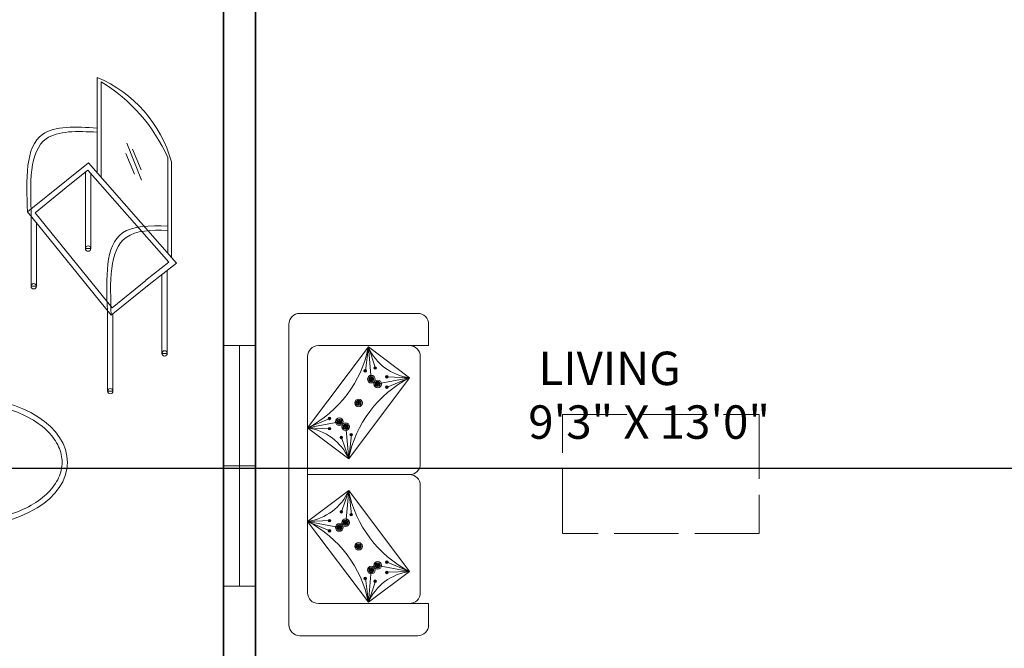
# Model space of a CAD drawing. Units: inches. Extents: x -61 to 1599, y -1316 to 257.
# Tile 19 of 204: x 76 to 259, y -907 to -790. Entities that reach past the tile are written whole.
import ezdxf

# ---------------------------------------------------------------- set-up
doc = ezdxf.new("R2010")
doc.units = ezdxf.units.IN
doc.header["$MEASUREMENT"] = 0
doc.linetypes.add('ACAD_ISO02W100', pattern=[15, 12, -3])
for name, color, linetype, lineweight in [('A-ANNO-DIMS', 2, 'Continuous', 18), ('A-AREA-IDEN', 1, 'Continuous', 18), ('A-FURN-LOW', 83, 'ACAD_ISO02W100', 18), ('FURNITURE', 83, 'Continuous', 18), ('WALLS', 4, 'Continuous', 35), ('WINDOWS', 220, 'Continuous', 18)]:
    doc.layers.add(name, color=color, linetype=linetype, lineweight=lineweight)
doc.layers.add('FUR', color=83, linetype='Continuous')
doc.styles.get("Standard").update_dxf_attribs({"font": 'arial.ttf'})
doc.dimstyles.get("Standard").update_dxf_attribs({"dimtxt": 0.18, "dimasz": 0.18, "dimexe": 0.18, "dimexo": 0.0625, "dimgap": 0.09, "dimtad": 0, "dimtih": 1, "dimtoh": 1, "dimdec": 0, "dimzin": 0, "dimdsep": 46, "dimlunit": 3, "dimtxsty": 'Standard', "dimcen": 0.09, "dimadec": 0, "dimazin": 0, "dimtfac": 1, "dimtdec": 0, "dimtofl": 0, "dimtmove": 0, "dimatfit": 3, "dimfxl": 1, "dimtolj": 1, "dimtzin": 0, "dimarcsym": 0})

# ---------------------------------------------------------------- blocks, each defined once
blk = doc.blocks.new('WIN-45IN')
for p, q in [((0, 44.83), (6, 44.83)), ((0, 0), (6, 0))]:
    blk.add_line(p, q)
for points in [[(6, 44.83), (3, 44.83), (3, 22.42), (6, 22.42)], [(3, 22.42), (0, 22.42), (0, 0), (3, 0)]]:
    blk.add_lwpolyline(points, close=True)
blk = doc.blocks.new('LOUNGE-CHAIR')
for p, q in [((14.76, 41.14), (14.76, 58.89)), ((14.04, 40.33), (14.04, 58.08)), ((6.52, 39.78), (9.29, 46.65)), ((6.58, 41.68), (8.18, 45.54)), ((7.84, 40.87), (9.45, 44.74)), ((0, 24.35), (16.38, 42.98)), ((0.97, 25.45), (0.97, 43.2)), ((0.97, 25.45), (0.97, 43.2)), ((1.64, 26.22), (1.64, 43.97)), ((16.38, 42.98), (20.51, 39.74)), ((16.97, 42.52), (16.97, 42.52)), ((1.45, 24.49), (16.5, 41.61)), ((15.97, 27.05), (15.97, 41.01)), ((16.5, 41.61), (19.89, 38.96)), ((16.97, 27.05), (16.97, 41.25)), ((19.88, 38.97), (26.35, 33.72)), ((20.51, 39.74), (27.76, 33.87)), ((12.02, 16.03), (26.35, 33.72)), ((12.16, 14.63), (27.76, 33.87)), ((27.1, 20.02), (27.1, 33.05)), ((26.1, 20.02), (26.1, 31.82)), ((16.97, 27.05), (15.97, 27.05)), ((0, 24.35), (5.1, 20.35)), ((1.45, 24.49), (5.72, 21.14)), ((0.75, 23.69), (0.79, 23.74)), ((1.73, 7.53), (1.73, 23)), ((2.73, 7.53), (2.73, 22.21)), ((5.1, 20.35), (12.16, 14.63)), ((5.73, 21.13), (12.02, 16.03)), ((27.1, 20.02), (26.1, 20.02)), ((11.85, 0.5), (11.85, 14.88)), ((12.85, 0.5), (12.85, 15.48)), ((2.73, 7.53), (1.73, 7.53)), ((12.85, 0.5), (11.85, 0.5))]:
    blk.add_line(p, q)
for centre in [(16.47, 27.05), (26.6, 20.02), (2.23, 7.53), (12.35, 0.5)]:
    blk.add_circle(centre, 0.5)
for centre, radius, start, end in [((23.93, 36.92), 23.8, 112.6586, 164.6996), ((30.25, 31.33), 31.28, 121.203, 156.1552)]:
    blk.add_arc(centre, radius, start, end)
for points, knots in [([(14.76, 49.49), (18.73, 49.7), (28.38, 50.23), (27.99, 39.93), (27.76, 33.87)], [0, 0, 0, 0, 10.281855, 24.983674, 24.983674, 24.983674, 24.983674]), ([(14.76, 48.72), (18.48, 48.91), (27.65, 49.16), (27.27, 39.12), (27.05, 33.06), (27.04, 33.03), (27.04, 33.01), (27.04, 32.98)], [0.614676, 0.614676, 0.614676, 0.614676, 10.281855, 24.983674, 24.983674, 24.983674, 25.041855, 25.041855, 25.041855, 25.041855]), ([(1.64, 31.22), (4.99, 31.37), (13.47, 31.24), (13.11, 21.57), (12.88, 15.51)], [1.527723, 1.527723, 1.527723, 1.527723, 10.281855, 24.983674, 24.983674, 24.983674, 24.983674]), ([(1.64, 30.44), (4.72, 30.55), (12.75, 30.17), (12.39, 20.76), (12.17, 14.7), (12.16, 14.67), (12.16, 14.65), (12.16, 14.63)], [2.150702, 2.150702, 2.150702, 2.150702, 10.281855, 24.983674, 24.983674, 24.983674, 25.041855, 25.041855, 25.041855, 25.041855])]:
    blk.add_open_spline(points, degree=3, knots=knots)
blk = doc.blocks.new('SIDE-TABLE-OVAL')
blk.add_ellipse((18.95, 11.99), major_axis=(-18.95, 0.16), ratio=0.632617)
blk.add_open_spline([(1, 12.14), (0.99, 11.17), (1.2, 10.2), (2.05, 8.28), (2.69, 7.34), (4.41, 5.58), (5.48, 4.76), (7.96, 3.32), (9.37, 2.71), (12.41, 1.74), (14.05, 1.4), (17.41, 1), (19.13, 0.95), (22.53, 1.15), (24.2, 1.41), (27.36, 2.19), (28.84, 2.73), (31.49, 4.02), (32.66, 4.78), (34.59, 6.45), (35.35, 7.36), (36.44, 9.24), (36.76, 10.2), (36.97, 12.14), (36.87, 13.11), (36.22, 15.04), (35.67, 16), (34.15, 17.81), (33.17, 18.67), (30.85, 20.19), (29.51, 20.86), (26.58, 21.94), (24.98, 22.36), (21.67, 22.89), (19.95, 23.01), (16.54, 22.94), (14.84, 22.76), (11.61, 22.1), (10.07, 21.63), (7.28, 20.44), (6.03, 19.73), (3.92, 18.13), (3.06, 17.25), (1.78, 15.4), (1.35, 14.44), (1.05, 13.03), (1, 12.59), (1, 12.14)], degree=3, knots=[0, 0, 0, 0, 0.279765, 0.279765, 0.559529, 0.559529, 0.839294, 0.839294, 1.119059, 1.119059, 1.398823, 1.398823, 1.678588, 1.678588, 1.958353, 1.958353, 2.238118, 2.238118, 2.517882, 2.517882, 2.797647, 2.797647, 3.077412, 3.077412, 3.357176, 3.357176, 3.636941, 3.636941, 3.916706, 3.916706, 4.19647, 4.19647, 4.476235, 4.476235, 4.756, 4.756, 5.035764, 5.035764, 5.315529, 5.315529, 5.595294, 5.595294, 5.875058, 5.875058, 6.154823, 6.154823, 6.283185, 6.283185, 6.283185, 6.283185])
blk = doc.blocks.new('*U160')
at = {"layer": 'FUR'}
blk.add_open_spline([(0, 0.08), (-0.03, 0.05), (-0.1, -0.02), (0.08, -0.02), (0.02, -0.06), (0, -0.08)], degree=3, knots=[0, 0, 0, 0, 0.0954578, 0.1898773, 0.2470677, 0.2470677, 0.2470677, 0.2470677], dxfattribs=at)
blk = doc.blocks.new('*U161')
at = {"layer": 'FUR', "transparency": 16777216}
for p, rotation in [((222.17, -79.98), 60), ((222.18, -80.06), 120), ((222.31, -79.97), 300), ((222.25, -80.09), 180), ((222.32, -80.05), 240)]:
    blk.add_blockref('*U160', p, dxfattribs=dict(at, rotation=rotation))
blk.add_blockref('*U160', (222.24, -79.93), dxfattribs=at)
blk = doc.blocks.new('*U172')
at = {"layer": 'FUR'}
blk.add_open_spline([(0, 0.08), (-0.03, 0.05), (-0.1, -0.02), (0.08, -0.02), (0.02, -0.06), (0, -0.08)], degree=3, knots=[0, 0, 0, 0, 0.0954578, 0.1898773, 0.2470677, 0.2470677, 0.2470677, 0.2470677], dxfattribs=at)
blk = doc.blocks.new('*U173')
at = {"layer": 'FUR', "transparency": 16777216}
for p, rotation in [((222.17, -79.98), 60), ((222.18, -80.06), 120), ((222.31, -79.97), 300), ((222.25, -80.09), 180), ((222.32, -80.05), 240)]:
    blk.add_blockref('*U172', p, dxfattribs=dict(at, rotation=rotation))
blk.add_blockref('*U172', (222.24, -79.93), dxfattribs=at)
blk = doc.blocks.new('*U186')
at = {"layer": 'FUR'}
blk.add_open_spline([(0, 0.08), (-0.03, 0.05), (-0.1, -0.02), (0.08, -0.02), (0.02, -0.06), (0, -0.08)], degree=3, knots=[0, 0, 0, 0, 0.0954578, 0.1898773, 0.2470677, 0.2470677, 0.2470677, 0.2470677], dxfattribs=at)
blk = doc.blocks.new('*U187')
at = {"layer": 'FUR', "transparency": 16777216}
for p, rotation in [((222.17, -79.98), 60), ((222.18, -80.06), 120), ((222.31, -79.97), 300), ((222.25, -80.09), 180), ((222.32, -80.05), 240)]:
    blk.add_blockref('*U186', p, dxfattribs=dict(at, rotation=rotation))
blk.add_blockref('*U186', (222.24, -79.93), dxfattribs=at)
blk = doc.blocks.new('*U198')
at = {"layer": 'FUR'}
blk.add_open_spline([(0, 0.08), (-0.03, 0.05), (-0.1, -0.02), (0.08, -0.02), (0.02, -0.06), (0, -0.08)], degree=3, knots=[0, 0, 0, 0, 0.0954578, 0.1898773, 0.2470677, 0.2470677, 0.2470677, 0.2470677], dxfattribs=at)
blk = doc.blocks.new('*U199')
at = {"layer": 'FUR', "transparency": 16777216}
for p, rotation in [((222.17, -79.98), 60), ((222.18, -80.06), 120), ((222.31, -79.97), 300), ((222.25, -80.09), 180), ((222.32, -80.05), 240)]:
    blk.add_blockref('*U198', p, dxfattribs=dict(at, rotation=rotation))
blk.add_blockref('*U198', (222.24, -79.93), dxfattribs=at)
blk = doc.blocks.new('*U184')
at = {"layer": 'FUR'}
blk.add_open_spline([(0.01, 0.24), (-0.09, 0.14), (-0.29, -0.05), (0.22, -0.05), (0.07, -0.19), (0.01, -0.24)], degree=3, knots=[0, 0, 0, 0, 0.2846533, 0.5662105, 0.736751, 0.736751, 0.736751, 0.736751], dxfattribs=at)
blk = doc.blocks.new('*U159')
at = {"layer": 'FUR', "transparency": 16777216}
for p, rotation in [((662.52, -238.49), 60), ((662.93, -238.46), 300), ((662.53, -238.73), 120), ((662.74, -238.83), 180), ((662.94, -238.7), 240)]:
    blk.add_blockref('*U184', p, dxfattribs=dict(at, rotation=rotation))
blk.add_blockref('*U184', (662.72, -238.36), dxfattribs=at)
blk = doc.blocks.new('*U210')
at = {"layer": 'FUR'}
blk.add_open_spline([(0.01, 0.24), (-0.09, 0.14), (-0.29, -0.05), (0.22, -0.05), (0.07, -0.19), (0.01, -0.24)], degree=3, knots=[0, 0, 0, 0, 0.2846533, 0.5662105, 0.736751, 0.736751, 0.736751, 0.736751], dxfattribs=at)
blk = doc.blocks.new('*U185')
at = {"layer": 'FUR', "transparency": 16777216}
for p, rotation in [((662.52, -238.49), 60), ((662.93, -238.46), 300), ((662.53, -238.73), 120), ((662.74, -238.83), 180), ((662.94, -238.7), 240)]:
    blk.add_blockref('*U210', p, dxfattribs=dict(at, rotation=rotation))
blk.add_blockref('*U210', (662.72, -238.36), dxfattribs=at)
blk = doc.blocks.new('*U174')
at = {"layer": 'FUR'}
blk.add_open_spline([(0, 0.08), (-0.03, 0.05), (-0.1, -0.02), (0.08, -0.02), (0.02, -0.06), (0, -0.08)], degree=3, knots=[0, 0, 0, 0, 0.0954578, 0.1898773, 0.2470677, 0.2470677, 0.2470677, 0.2470677], dxfattribs=at)
blk = doc.blocks.new('*U175')
at = {"layer": 'FUR', "transparency": 16777216}
for p, rotation in [((222.17, -79.98), 60), ((222.18, -80.06), 120), ((222.31, -79.97), 300), ((222.25, -80.09), 180), ((222.32, -80.05), 240)]:
    blk.add_blockref('*U174', p, dxfattribs=dict(at, rotation=rotation))
blk.add_blockref('*U174', (222.24, -79.93), dxfattribs=at)
blk = doc.blocks.new('*U200')
at = {"layer": 'FUR'}
blk.add_open_spline([(0, 0.08), (-0.03, 0.05), (-0.1, -0.02), (0.08, -0.02), (0.02, -0.06), (0, -0.08)], degree=3, knots=[0, 0, 0, 0, 0.0954578, 0.1898773, 0.2470677, 0.2470677, 0.2470677, 0.2470677], dxfattribs=at)
blk = doc.blocks.new('*U201')
at = {"layer": 'FUR', "transparency": 16777216}
for p, rotation in [((222.17, -79.98), 60), ((222.18, -80.06), 120), ((222.31, -79.97), 300), ((222.25, -80.09), 180), ((222.32, -80.05), 240)]:
    blk.add_blockref('*U200', p, dxfattribs=dict(at, rotation=rotation))
blk.add_blockref('*U200', (222.24, -79.93), dxfattribs=at)
blk = doc.blocks.new('*U168')
at = {"layer": 'FUR'}
blk.add_open_spline([(0.01, 0.24), (-0.09, 0.14), (-0.29, -0.05), (0.22, -0.05), (0.07, -0.19), (0.01, -0.24)], degree=3, knots=[0, 0, 0, 0, 0.2846533, 0.5662105, 0.736751, 0.736751, 0.736751, 0.736751], dxfattribs=at)
blk = doc.blocks.new('*U169')
at = {"layer": 'FUR', "transparency": 16777216}
for p, rotation in [((662.52, -238.49), 60), ((662.93, -238.46), 300), ((662.53, -238.73), 120), ((662.74, -238.83), 180), ((662.94, -238.7), 240)]:
    blk.add_blockref('*U168', p, dxfattribs=dict(at, rotation=rotation))
blk.add_blockref('*U168', (662.72, -238.36), dxfattribs=at)
blk = doc.blocks.new('*U194')
at = {"layer": 'FUR'}
blk.add_open_spline([(0.01, 0.24), (-0.09, 0.14), (-0.29, -0.05), (0.22, -0.05), (0.07, -0.19), (0.01, -0.24)], degree=3, knots=[0, 0, 0, 0, 0.2846533, 0.5662105, 0.736751, 0.736751, 0.736751, 0.736751], dxfattribs=at)
blk = doc.blocks.new('*U195')
at = {"layer": 'FUR', "transparency": 16777216}
for p, rotation in [((662.52, -238.49), 60), ((662.93, -238.46), 300), ((662.53, -238.73), 120), ((662.74, -238.83), 180), ((662.94, -238.7), 240)]:
    blk.add_blockref('*U194', p, dxfattribs=dict(at, rotation=rotation))
blk.add_blockref('*U194', (662.72, -238.36), dxfattribs=at)
blk = doc.blocks.new('*U176')
at = {"layer": 'FUR'}
blk.add_open_spline([(0, 0.08), (-0.03, 0.05), (-0.1, -0.02), (0.08, -0.02), (0.02, -0.06), (0, -0.08)], degree=3, knots=[0, 0, 0, 0, 0.0954578, 0.1898773, 0.2470677, 0.2470677, 0.2470677, 0.2470677], dxfattribs=at)
blk = doc.blocks.new('*U177')
at = {"layer": 'FUR', "transparency": 16777216}
for p, rotation in [((222.17, -79.98), 60), ((222.18, -80.06), 120), ((222.31, -79.97), 300), ((222.25, -80.09), 180), ((222.32, -80.05), 240)]:
    blk.add_blockref('*U176', p, dxfattribs=dict(at, rotation=rotation))
blk.add_blockref('*U176', (222.24, -79.93), dxfattribs=at)
blk = doc.blocks.new('*U202')
at = {"layer": 'FUR'}
blk.add_open_spline([(0, 0.08), (-0.03, 0.05), (-0.1, -0.02), (0.08, -0.02), (0.02, -0.06), (0, -0.08)], degree=3, knots=[0, 0, 0, 0, 0.0954578, 0.1898773, 0.2470677, 0.2470677, 0.2470677, 0.2470677], dxfattribs=at)
blk = doc.blocks.new('*U203')
at = {"layer": 'FUR', "transparency": 16777216}
for p, rotation in [((222.17, -79.98), 60), ((222.18, -80.06), 120), ((222.31, -79.97), 300), ((222.25, -80.09), 180), ((222.32, -80.05), 240)]:
    blk.add_blockref('*U202', p, dxfattribs=dict(at, rotation=rotation))
blk.add_blockref('*U202', (222.24, -79.93), dxfattribs=at)
blk = doc.blocks.new('*U170')
at = {"layer": 'FUR'}
blk.add_open_spline([(0.01, 0.24), (-0.09, 0.14), (-0.29, -0.05), (0.22, -0.05), (0.07, -0.19), (0.01, -0.24)], degree=3, knots=[0, 0, 0, 0, 0.2846533, 0.5662105, 0.736751, 0.736751, 0.736751, 0.736751], dxfattribs=at)
blk = doc.blocks.new('*U171')
at = {"layer": 'FUR', "transparency": 16777216}
for p, rotation in [((662.52, -238.49), 60), ((662.93, -238.46), 300), ((662.53, -238.73), 120), ((662.74, -238.83), 180), ((662.94, -238.7), 240)]:
    blk.add_blockref('*U170', p, dxfattribs=dict(at, rotation=rotation))
blk.add_blockref('*U170', (662.72, -238.36), dxfattribs=at)
blk = doc.blocks.new('*U196')
at = {"layer": 'FUR'}
blk.add_open_spline([(0.01, 0.24), (-0.09, 0.14), (-0.29, -0.05), (0.22, -0.05), (0.07, -0.19), (0.01, -0.24)], degree=3, knots=[0, 0, 0, 0, 0.2846533, 0.5662105, 0.736751, 0.736751, 0.736751, 0.736751], dxfattribs=at)
blk = doc.blocks.new('*U197')
at = {"layer": 'FUR', "transparency": 16777216}
for p, rotation in [((662.52, -238.49), 60), ((662.93, -238.46), 300), ((662.53, -238.73), 120), ((662.74, -238.83), 180), ((662.94, -238.7), 240)]:
    blk.add_blockref('*U196', p, dxfattribs=dict(at, rotation=rotation))
blk.add_blockref('*U196', (662.72, -238.36), dxfattribs=at)
blk = doc.blocks.new('*U164')
at = {"layer": 'FUR'}
blk.add_open_spline([(0, 0.08), (-0.03, 0.05), (-0.1, -0.02), (0.08, -0.02), (0.02, -0.06), (0, -0.08)], degree=3, knots=[0, 0, 0, 0, 0.0954578, 0.1898773, 0.2470677, 0.2470677, 0.2470677, 0.2470677], dxfattribs=at)
blk = doc.blocks.new('*U165')
at = {"layer": 'FUR', "transparency": 16777216}
for p, rotation in [((222.17, -79.98), 60), ((222.18, -80.06), 120), ((222.31, -79.97), 300), ((222.25, -80.09), 180), ((222.32, -80.05), 240)]:
    blk.add_blockref('*U164', p, dxfattribs=dict(at, rotation=rotation))
blk.add_blockref('*U164', (222.24, -79.93), dxfattribs=at)
blk = doc.blocks.new('*U190')
at = {"layer": 'FUR'}
blk.add_open_spline([(0, 0.08), (-0.03, 0.05), (-0.1, -0.02), (0.08, -0.02), (0.02, -0.06), (0, -0.08)], degree=3, knots=[0, 0, 0, 0, 0.0954578, 0.1898773, 0.2470677, 0.2470677, 0.2470677, 0.2470677], dxfattribs=at)
blk = doc.blocks.new('*U191')
at = {"layer": 'FUR', "transparency": 16777216}
for p, rotation in [((222.17, -79.98), 60), ((222.18, -80.06), 120), ((222.31, -79.97), 300), ((222.25, -80.09), 180), ((222.32, -80.05), 240)]:
    blk.add_blockref('*U190', p, dxfattribs=dict(at, rotation=rotation))
blk.add_blockref('*U190', (222.24, -79.93), dxfattribs=at)
blk = doc.blocks.new('*U183')
at = {"layer": 'FUR'}
blk.add_open_spline([(0.01, 0.24), (-0.09, 0.14), (-0.29, -0.05), (0.22, -0.05), (0.07, -0.19), (0.01, -0.24)], degree=3, knots=[0, 0, 0, 0, 0.2846533, 0.5662105, 0.736751, 0.736751, 0.736751, 0.736751], dxfattribs=at)
blk = doc.blocks.new('*U162')
at = {"layer": 'FUR', "transparency": 16777216}
for p, rotation in [((662.52, -238.49), 60), ((662.93, -238.46), 300), ((662.53, -238.73), 120), ((662.74, -238.83), 180), ((662.94, -238.7), 240)]:
    blk.add_blockref('*U183', p, dxfattribs=dict(at, rotation=rotation))
blk.add_blockref('*U183', (662.72, -238.36), dxfattribs=at)
blk = doc.blocks.new('*U209')
at = {"layer": 'FUR'}
blk.add_open_spline([(0.01, 0.24), (-0.09, 0.14), (-0.29, -0.05), (0.22, -0.05), (0.07, -0.19), (0.01, -0.24)], degree=3, knots=[0, 0, 0, 0, 0.2846533, 0.5662105, 0.736751, 0.736751, 0.736751, 0.736751], dxfattribs=at)
blk = doc.blocks.new('*U188')
at = {"layer": 'FUR', "transparency": 16777216}
for p, rotation in [((662.52, -238.49), 60), ((662.93, -238.46), 300), ((662.53, -238.73), 120), ((662.74, -238.83), 180), ((662.94, -238.7), 240)]:
    blk.add_blockref('*U209', p, dxfattribs=dict(at, rotation=rotation))
blk.add_blockref('*U209', (662.72, -238.36), dxfattribs=at)
blk = doc.blocks.new('*U182')
at = {"layer": 'FUR'}
blk.add_open_spline([(0, 0.08), (-0.03, 0.05), (-0.1, -0.02), (0.08, -0.02), (0.02, -0.06), (0, -0.08)], degree=3, knots=[0, 0, 0, 0, 0.0954578, 0.1898773, 0.2470677, 0.2470677, 0.2470677, 0.2470677], dxfattribs=at)
blk = doc.blocks.new('*U163')
at = {"layer": 'FUR', "transparency": 16777216}
for p, rotation in [((222.17, -79.98), 60), ((222.18, -80.06), 120), ((222.31, -79.97), 300), ((222.25, -80.09), 180), ((222.32, -80.05), 240)]:
    blk.add_blockref('*U182', p, dxfattribs=dict(at, rotation=rotation))
blk.add_blockref('*U182', (222.24, -79.93), dxfattribs=at)
blk = doc.blocks.new('*U208')
at = {"layer": 'FUR'}
blk.add_open_spline([(0, 0.08), (-0.03, 0.05), (-0.1, -0.02), (0.08, -0.02), (0.02, -0.06), (0, -0.08)], degree=3, knots=[0, 0, 0, 0, 0.0954578, 0.1898773, 0.2470677, 0.2470677, 0.2470677, 0.2470677], dxfattribs=at)
blk = doc.blocks.new('*U189')
at = {"layer": 'FUR', "transparency": 16777216}
for p, rotation in [((222.17, -79.98), 60), ((222.18, -80.06), 120), ((222.31, -79.97), 300), ((222.25, -80.09), 180), ((222.32, -80.05), 240)]:
    blk.add_blockref('*U208', p, dxfattribs=dict(at, rotation=rotation))
blk.add_blockref('*U208', (222.24, -79.93), dxfattribs=at)
blk = doc.blocks.new('*U166')
at = {"layer": 'FUR'}
blk.add_open_spline([(0.01, 0.24), (-0.09, 0.14), (-0.29, -0.05), (0.22, -0.05), (0.07, -0.19), (0.01, -0.24)], degree=3, knots=[0, 0, 0, 0, 0.2846533, 0.5662105, 0.736751, 0.736751, 0.736751, 0.736751], dxfattribs=at)
blk = doc.blocks.new('*U167')
at = {"layer": 'FUR', "transparency": 16777216}
for p, rotation in [((662.52, -238.49), 60), ((662.93, -238.46), 300), ((662.53, -238.73), 120), ((662.74, -238.83), 180), ((662.94, -238.7), 240)]:
    blk.add_blockref('*U166', p, dxfattribs=dict(at, rotation=rotation))
blk.add_blockref('*U166', (662.72, -238.36), dxfattribs=at)
blk = doc.blocks.new('*U192')
at = {"layer": 'FUR'}
blk.add_open_spline([(0.01, 0.24), (-0.09, 0.14), (-0.29, -0.05), (0.22, -0.05), (0.07, -0.19), (0.01, -0.24)], degree=3, knots=[0, 0, 0, 0, 0.2846533, 0.5662105, 0.736751, 0.736751, 0.736751, 0.736751], dxfattribs=at)
blk = doc.blocks.new('*U193')
at = {"layer": 'FUR', "transparency": 16777216}
for p, rotation in [((662.52, -238.49), 60), ((662.93, -238.46), 300), ((662.53, -238.73), 120), ((662.74, -238.83), 180), ((662.94, -238.7), 240)]:
    blk.add_blockref('*U192', p, dxfattribs=dict(at, rotation=rotation))
blk.add_blockref('*U192', (662.72, -238.36), dxfattribs=at)
blk = doc.blocks.new('*U178')
at = {"layer": 'FUR'}
blk.add_open_spline([(0, 0.08), (-0.03, 0.05), (-0.1, -0.02), (0.08, -0.02), (0.02, -0.06), (0, -0.08)], degree=3, knots=[0, 0, 0, 0, 0.0954578, 0.1898773, 0.2470677, 0.2470677, 0.2470677, 0.2470677], dxfattribs=at)
blk = doc.blocks.new('*U179')
at = {"layer": 'FUR', "transparency": 16777216}
for p, rotation in [((222.17, -79.98), 60), ((222.18, -80.06), 120), ((222.31, -79.97), 300), ((222.25, -80.09), 180), ((222.32, -80.05), 240)]:
    blk.add_blockref('*U178', p, dxfattribs=dict(at, rotation=rotation))
blk.add_blockref('*U178', (222.24, -79.93), dxfattribs=at)
blk = doc.blocks.new('*U180')
at = {"layer": 'FUR'}
blk.add_open_spline([(0, 0.08), (-0.03, 0.05), (-0.1, -0.02), (0.08, -0.02), (0.02, -0.06), (0, -0.08)], degree=3, knots=[0, 0, 0, 0, 0.0954578, 0.1898773, 0.2470677, 0.2470677, 0.2470677, 0.2470677], dxfattribs=at)
blk = doc.blocks.new('*U181')
at = {"layer": 'FUR', "transparency": 16777216}
for p, rotation in [((222.17, -79.98), 60), ((222.18, -80.06), 120), ((222.31, -79.97), 300), ((222.25, -80.09), 180), ((222.32, -80.05), 240)]:
    blk.add_blockref('*U180', p, dxfattribs=dict(at, rotation=rotation))
blk.add_blockref('*U180', (222.24, -79.93), dxfattribs=at)
blk = doc.blocks.new('*U204')
at = {"layer": 'FUR'}
blk.add_open_spline([(0, 0.08), (-0.03, 0.05), (-0.1, -0.02), (0.08, -0.02), (0.02, -0.06), (0, -0.08)], degree=3, knots=[0, 0, 0, 0, 0.0954578, 0.1898773, 0.2470677, 0.2470677, 0.2470677, 0.2470677], dxfattribs=at)
blk = doc.blocks.new('*U205')
at = {"layer": 'FUR', "transparency": 16777216}
for p, rotation in [((222.17, -79.98), 60), ((222.18, -80.06), 120), ((222.31, -79.97), 300), ((222.25, -80.09), 180), ((222.32, -80.05), 240)]:
    blk.add_blockref('*U204', p, dxfattribs=dict(at, rotation=rotation))
blk.add_blockref('*U204', (222.24, -79.93), dxfattribs=at)
blk = doc.blocks.new('*U206')
at = {"layer": 'FUR'}
blk.add_open_spline([(0, 0.08), (-0.03, 0.05), (-0.1, -0.02), (0.08, -0.02), (0.02, -0.06), (0, -0.08)], degree=3, knots=[0, 0, 0, 0, 0.0954578, 0.1898773, 0.2470677, 0.2470677, 0.2470677, 0.2470677], dxfattribs=at)
blk = doc.blocks.new('*U207')
at = {"layer": 'FUR', "transparency": 16777216}
for p, rotation in [((222.17, -79.98), 60), ((222.18, -80.06), 120), ((222.31, -79.97), 300), ((222.25, -80.09), 180), ((222.32, -80.05), 240)]:
    blk.add_blockref('*U206', p, dxfattribs=dict(at, rotation=rotation))
blk.add_blockref('*U206', (222.24, -79.93), dxfattribs=at)
blk = doc.blocks.new('SOFA-LOVESEAT')
for p, q in [((22.44, 54), (5.47, 54)), ((14.78, 53.75), (14.25, 49.29)), ((14.78, 53.75), (15.33, 47.76)), ((14.78, 53.75), (16.08, 49.82)), ((22.44, 54), (26, 54)), ((3.47, 8), (3.47, 52)), ((24.44, 52), (24.44, 32)), ((16.03, 49.84), (15.87, 49.84)), ((16.03, 49.84), (16.19, 49.84)), ((14.2, 49.3), (14.04, 49.3)), ((14.2, 49.3), (14.36, 49.3)), ((15.33, 47.76), (14.86, 47.76)), ((15.33, 47.76), (15.81, 47.76)), ((22.42, 48.01), (16.51, 46.87)), ((18.23, 48.19), (18.07, 48.19)), ((18.23, 48.19), (18.39, 48.19)), ((22.42, 48.01), (18.28, 48.17)), ((22.42, 48.01), (18.28, 46.26)), ((16.51, 46.87), (16.03, 46.87)), ((16.51, 46.87), (16.99, 46.87)), ((18.23, 46.28), (18.07, 46.28)), ((18.23, 46.28), (18.39, 46.28)), ((12.95, 43.35), (12.47, 43.35)), ((12.95, 43.35), (13.42, 43.35)), ((3.47, 38.69), (7.61, 40.44)), ((7.56, 40.46), (7.4, 40.46)), ((7.56, 40.46), (7.72, 40.46)), ((3.47, 38.69), (9.38, 39.83)), ((3.47, 38.69), (7.61, 38.53)), ((7.56, 38.55), (7.4, 38.55)), ((7.56, 38.55), (7.72, 38.55)), ((9.38, 39.83), (8.9, 39.83)), ((9.38, 39.83), (9.86, 39.83)), ((10.56, 38.94), (10.08, 38.94)), ((11.12, 32.95), (10.56, 38.94)), ((10.56, 38.94), (11.04, 38.94)), ((9.76, 36.9), (9.6, 36.9)), ((9.76, 36.9), (9.92, 36.9)), ((11.12, 32.95), (9.81, 36.88)), ((11.12, 32.95), (11.64, 37.41)), ((11.59, 37.43), (11.43, 37.43)), ((11.59, 37.43), (11.75, 37.43)), ((22.44, 30), (3.47, 30)), ((22.44, 30), (22.44, 30)), ((24.44, 8), (24.44, 28)), ((11.12, 27.03), (9.81, 23.09)), ((11.12, 27.03), (10.56, 21.03)), ((11.12, 27.03), (11.64, 22.56)), ((9.76, 23.07), (9.6, 23.07)), ((9.76, 23.07), (9.92, 23.07)), ((11.59, 22.54), (11.43, 22.54)), ((11.59, 22.54), (11.75, 22.54)), ((3.47, 21.29), (7.61, 21.44)), ((3.47, 21.29), (9.38, 20.15)), ((3.47, 21.29), (7.61, 19.54)), ((7.56, 21.42), (7.4, 21.42)), ((7.56, 21.42), (7.72, 21.42)), ((10.56, 21.03), (10.08, 21.03)), ((10.56, 21.03), (11.04, 21.03)), ((7.56, 19.52), (7.4, 19.52)), ((7.56, 19.52), (7.72, 19.52)), ((9.38, 20.15), (8.9, 20.15)), ((9.38, 20.15), (9.86, 20.15)), ((12.95, 16.62), (12.47, 16.62)), ((12.95, 16.62), (13.42, 16.62)), ((16.51, 13.1), (16.03, 13.1)), ((22.42, 11.96), (16.51, 13.1)), ((16.51, 13.1), (16.99, 13.1)), ((18.23, 13.69), (18.07, 13.69)), ((18.23, 13.69), (18.39, 13.69)), ((22.42, 11.96), (18.28, 13.71)), ((14.78, 6.22), (15.33, 12.22)), ((15.33, 12.22), (14.86, 12.22)), ((15.33, 12.22), (15.81, 12.22)), ((18.23, 11.79), (18.07, 11.79)), ((18.23, 11.79), (18.39, 11.79)), ((22.42, 11.96), (18.28, 11.81)), ((14.2, 10.67), (14.04, 10.67)), ((14.2, 10.67), (14.36, 10.67)), ((14.78, 6.22), (14.25, 10.69)), ((14.78, 6.22), (16.08, 10.16)), ((16.03, 10.14), (15.87, 10.14)), ((16.03, 10.14), (16.19, 10.14)), ((22.44, 6), (5.47, 6)), ((22.44, 6), (26, 6))]:
    blk.add_line(p, q)
blk.add_lwpolyline([(26, 6), (26, 2, -0.414214), (24, 0), (2, 0, -0.414214), (0, 2), (0, 58, -0.414213), (2, 60), (24, 60, -0.414214), (26, 58), (26, 54)], format="xyb")
for points in [[(11.12, 32.95), (22.42, 48.01), (14.78, 53.75), (3.47, 38.69)], [(11.12, 27.03), (22.42, 11.96), (14.78, 6.22), (3.47, 21.29)]]:
    blk.add_lwpolyline(points, close=True)
for centre, radius in [((14.2, 49.3), 0.238), ((16.03, 49.84), 0.238), ((16.03, 49.84), 0.16), ((14.2, 49.3), 0.16), ((15.33, 47.76), 0.71), ((15.33, 47.76), 0.476), ((18.23, 48.19), 0.238), ((18.23, 48.19), 0.16), ((16.51, 46.87), 0.71), ((16.51, 46.87), 0.476), ((18.23, 46.28), 0.238), ((18.23, 46.28), 0.16), ((12.95, 43.35), 0.71), ((12.95, 43.35), 0.476), ((7.56, 40.46), 0.238), ((7.56, 40.46), 0.16), ((9.38, 39.83), 0.71), ((7.56, 38.55), 0.238), ((7.56, 38.55), 0.16), ((9.38, 39.83), 0.476), ((10.56, 38.94), 0.71), ((10.56, 38.94), 0.476), ((9.76, 36.9), 0.238), ((9.76, 36.9), 0.16), ((11.59, 37.43), 0.238), ((11.59, 37.43), 0.16), ((9.76, 23.07), 0.238), ((9.76, 23.07), 0.16), ((11.59, 22.54), 0.238), ((11.59, 22.54), 0.16), ((7.56, 21.42), 0.238), ((7.56, 21.42), 0.16), ((9.38, 20.15), 0.71), ((9.38, 20.15), 0.476), ((10.56, 21.03), 0.71), ((10.56, 21.03), 0.476), ((7.56, 19.52), 0.238), ((7.56, 19.52), 0.16), ((12.95, 16.62), 0.71), ((12.95, 16.62), 0.476), ((15.33, 12.22), 0.71), ((16.51, 13.1), 0.71), ((16.51, 13.1), 0.476), ((18.23, 13.69), 0.238), ((18.23, 13.69), 0.16), ((15.33, 12.22), 0.476), ((18.23, 11.79), 0.238), ((18.23, 11.79), 0.16), ((14.2, 10.67), 0.238), ((14.2, 10.67), 0.16), ((16.03, 10.14), 0.238), ((16.03, 10.14), 0.16)]:
    blk.add_circle(centre, radius)
for centre, radius, start, end in [((5.47, 52), 2, 90, 180), ((-6.54, 57.97), 21.73, 297.4317, 348.7956), ((23.75, 57.74), 9.82, 203.9742, 262.253), ((22.44, 52), 2, 0, 90), ((32.43, 28.73), 21.73, 117.4317, 168.7956), ((2.15, 28.96), 9.82, 23.9742, 82.253), ((22.44, 32), 2, 270, 0), ((22.44, 28), 2, 0, 90), ((2.15, 31.01), 9.82, 277.747, 336.0258), ((32.43, 31.25), 21.73, 191.2044, 242.5684), ((-6.54, 2), 21.73, 11.2044, 62.5684), ((23.75, 2.23), 9.82, 97.747, 156.0258), ((5.47, 8), 2, 180, 270), ((22.44, 8), 2, 270, 0)]:
    blk.add_arc(centre, radius, start, end)
at = {"xscale": -1, "rotation": 90.00003000000098}
for name, p in [('*U189', (-63.98, 272.08)), ('*U191', (-65.81, 271.55)), ('*U188', (-223.26, 710.49)), ('*U205', (-61.78, 270.43)), ('*U193', (-222.08, 709.6)), ('*U207', (-61.78, 268.53)), ('*U197', (-225.65, 706.08)), ('*U187', (-72.45, 262.7)), ('*U185', (-229.21, 702.56)), ('*U199', (-72.45, 260.8)), ('*U195', (-228.03, 701.67)), ('*U201', (-70.25, 259.15)), ('*U203', (-68.43, 259.68))]:
    blk.add_blockref(name, p, dxfattribs=at)
at = {"rotation": 90}
for name, p in [('*U175', (-70.25, -199.17)), ('*U177', (-68.43, -199.7)), ('*U173', (-72.45, -200.82)), ('*U159', (-229.21, -642.58)), ('*U169', (-228.03, -641.7)), ('*U161', (-72.45, -202.73)), ('*U171', (-225.65, -646.11)), ('*U167', (-222.08, -649.63)), ('*U181', (-61.78, -208.55)), ('*U162', (-223.26, -650.51)), ('*U179', (-61.78, -210.46)), ('*U165', (-65.81, -211.58)), ('*U163', (-63.98, -212.11))]:
    blk.add_blockref(name, p, dxfattribs=at)
blk = doc.blocks.new('*D687')
at = {"layer": 'A-ANNO-DIMS', "color": 0, "lineweight": -2, "transparency": 16777216}
for p, q in [((289.42, 181.68), (-61.08, 181.68)), ((-60.9, 181.5), (-60.9, -528.95)), ((-60.9, -1239.76), (-60.9, -529.32)), ((319.64, -1239.94), (-61.08, -1239.94))]:
    blk.add_line(p, q, dxfattribs=at)
at = {"layer": 'A-ANNO-DIMS', "color": 0, "transparency": 16777216}
for points in [[(-60.93, 181.5), (-60.87, 181.5), (-60.9, 181.68)], [(-60.93, -1239.76), (-60.87, -1239.76), (-60.9, -1239.94)]]:
    blk.add_solid(points, dxfattribs=at)
at = {"layer": 'DEFPOINTS', "color": 0, "transparency": 16777216}
for p in [(289.48, 181.68), (-60.9, -1239.94), (319.7, -1239.94)]:
    blk.add_point(p, dxfattribs=at)
at = {"layer": 'A-ANNO-DIMS', "color": 0, "transparency": 16777216, "insert": (-60.9, -529.13), "char_height": 0.18, "attachment_point": 5}
blk.add_mtext('\\A1;1421.6', dxfattribs=at)
blk = doc.blocks.new('*D696')
at = {"layer": 'A-ANNO-DIMS', "color": 0, "lineweight": -2, "transparency": 16777216}
for p, q in [((690.64, -873.17), (-61.08, -873.17)), ((-60.9, -873.35), (-60.9, -1025.8)), ((-60.9, -1178.61), (-60.9, -1026.16)), ((690.64, -1178.79), (-61.08, -1178.79))]:
    blk.add_line(p, q, dxfattribs=at)
at = {"layer": 'A-ANNO-DIMS', "color": 0, "transparency": 16777216}
for points in [[(-60.93, -873.35), (-60.87, -873.35), (-60.9, -873.17)], [(-60.93, -1178.61), (-60.87, -1178.61), (-60.9, -1178.79)]]:
    blk.add_solid(points, dxfattribs=at)
at = {"layer": 'DEFPOINTS', "color": 0, "transparency": 16777216}
for p in [(-60.9, -873.17), (690.7, -873.17), (690.7, -1178.79)]:
    blk.add_point(p, dxfattribs=at)
at = {"layer": 'A-ANNO-DIMS', "color": 0, "transparency": 16777216, "insert": (-60.9, -1025.98), "char_height": 0.18, "attachment_point": 5}
blk.add_mtext('\\A1;305.6', dxfattribs=at)

msp = doc.modelspace()

# ---------------------------------------------------------------- linework, layer by layer
at = {"layer": 'A-FURN-LOW'}
msp.add_lwpolyline([(213.4399, -885.2801), (176.794, -885.2801), (176.794, -863.1137), (213.4399, -863.1137)], close=True, dxfattribs=at)
at = {"layer": 'WALLS'}
for p, q in [((113.7028, -943.9446), (113.7028, -787.9446)), ((119.7028, -943.9446), (119.7028, -787.9446))]:
    msp.add_line(p, q, dxfattribs=at)

# ---------------------------------------------------------------- block references
at = {"layer": 'FURNITURE', "extrusion": (0, 0, -1), "zscale": -1}
msp.add_blockref('LOUNGE-CHAIR', (-104.9843, -859.2896), dxfattribs=at)
at = {"layer": 'FURNITURE'}
for name, p in [('SOFA-LOVESEAT', (125.901, -904.3167)), ('SIDE-TABLE-OVAL', (46.761, -883.9187))]:
    msp.add_blockref(name, p, dxfattribs=at)
at = {"layer": 'WINDOWS'}
msp.add_blockref('WIN-45IN', (113.703, -895.1197), dxfattribs=at)

# ---------------------------------------------------------------- texts
at = {"layer": 'A-AREA-IDEN'}
for s, height, p in [('   LIVING', 6.22364, (166.6485, -857.6553)), ('  9\'3" X 13\'0"', 6.223643, (166.6485, -867.653))]:
    msp.add_text(s, height=height, dxfattribs=at).set_placement(p)

# ---------------------------------------------------------------- dimensions: what is measured, and where the dimension line sits
at = {"layer": 'A-ANNO-DIMS'}
for base, p1, p2, picture, middle in [((-60.8972, -1239.9446), (289.4807, 181.6771), (319.7028, -1239.9446), '*D687', (-60.8972, -529.1337)), ((-60.8972, -873.169), (690.7028, -1178.7933), (690.7028, -873.169), '*D696', (-60.8972, -1025.9812))]:
    dim = msp.add_linear_dim(base=base, p1=p1, p2=p2, angle=90, dimstyle='Standard', override={"dimdec": 1, "dimlfac": 1, "dimrnd": 0, "dimzin": 0, "dimdsep": 46, "dimlunit": 2}, dxfattribs=at)
    dim.commit()
    dim.dimension.update_dxf_attribs({"geometry": picture, "text_midpoint": middle})

doc.saveas('drawing.dxf')
